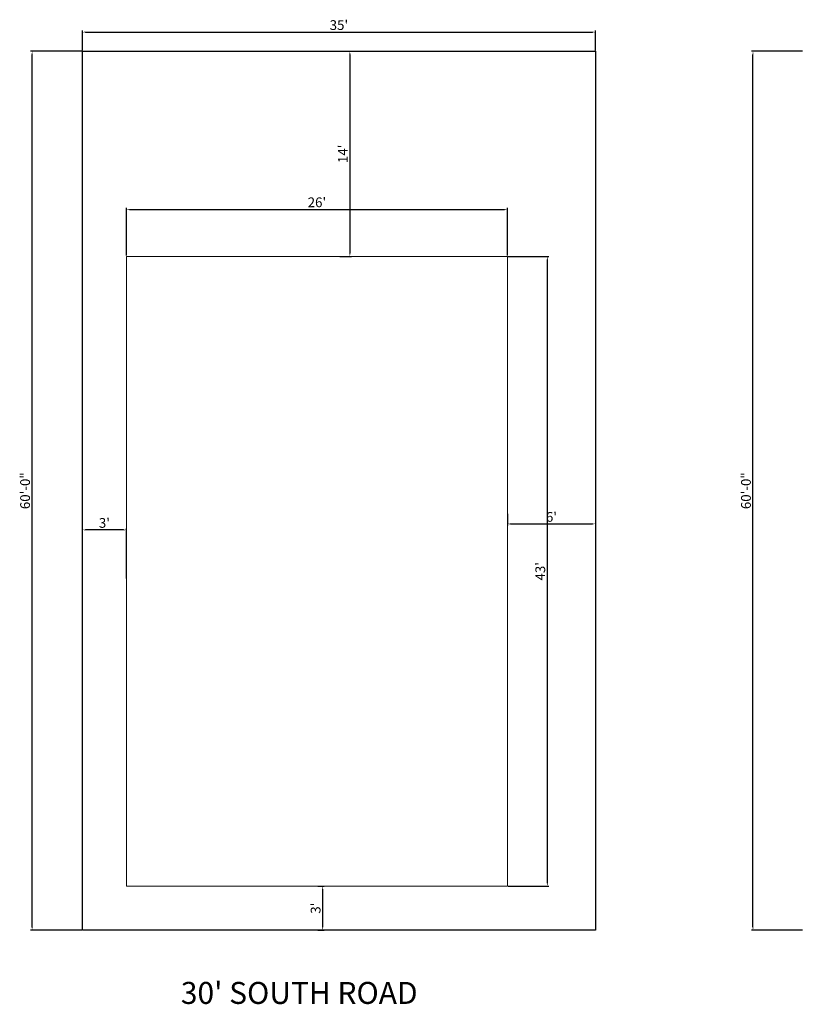
# Model space of a CAD drawing. Units: inches. Extents: x 538 to 2251, y 1112 to 1944.
# Tile 1 of 2: x 538 to 1179, y 1112 to 1918. Entities that reach past the tile are written whole.
import ezdxf

# ---------------------------------------------------------------- set-up
doc = ezdxf.new("R2010")
doc.units = ezdxf.units.IN
for name, color, linetype, lineweight in [('A-FLOR-OTLN', 7, 'Continuous', 18), ('C-PROP', 7, 'Continuous', 25), ('DIMENSIONS', 6, 'Continuous', 18), ('TEXT', 7, 'Continuous', 25)]:
    doc.layers.add(name, color=color, linetype=linetype, lineweight=lineweight)
doc.styles.get("Standard").update_dxf_attribs({"font": 'arial.ttf'})
doc.dimstyles.new('ISO-25', dxfattribs={"dimtxt": 8, "dimasz": 2.5, "dimexe": 1.25, "dimexo": 0.625, "dimtad": 1, "dimdec": 1, "dimlunit": 4, "dimtxsty": 'Standard', "dimcen": 2.5, "dimadec": 0, "dimazin": 0, "dimtfac": 1, "dimtdec": 1, "dimtmove": 0, "dimatfit": 3, "dimfxl": 1, "dimarcsym": 0})

# ---------------------------------------------------------------- blocks, each defined once
blk = doc.blocks.new('*D1')
at = {"layer": 'Defpoints', "color": 0, "transparency": 16777216}
for p in [(1008.95, 1908.31), (588.95, 1892.58), (1008.95, 1892.58)]:
    blk.add_point(p, dxfattribs=at)
at = {"layer": 'DIMENSIONS', "color": 0, "lineweight": -2, "transparency": 16777216}
for p, q in [((588.95, 1893.21), (588.95, 1909.56)), ((591.45, 1908.31), (1006.45, 1908.31)), ((1008.95, 1893.21), (1008.95, 1909.56))]:
    blk.add_line(p, q, dxfattribs=at)
at = {"layer": 'DIMENSIONS', "color": 0, "transparency": 16777216}
for points in [[(591.45, 1908.73), (591.45, 1907.9), (588.95, 1908.31)], [(1006.45, 1908.73), (1006.45, 1907.9), (1008.95, 1908.31)]]:
    blk.add_solid(points, dxfattribs=at)
at = {"layer": 'DIMENSIONS', "color": 0, "transparency": 16777216, "insert": (798.95, 1913.02), "char_height": 8, "attachment_point": 5}
blk.add_mtext("35'", dxfattribs=at)
blk = doc.blocks.new('*D2')
at = {"layer": 'Defpoints', "color": 0, "transparency": 16777216}
for p in [(936.95, 1763.11), (624.95, 1724.58), (936.95, 1724.58)]:
    blk.add_point(p, dxfattribs=at)
at = {"layer": 'DIMENSIONS', "color": 0, "lineweight": -2, "transparency": 16777216}
for p, q in [((624.95, 1725.21), (624.95, 1764.36)), ((627.45, 1763.11), (934.45, 1763.11)), ((936.95, 1725.21), (936.95, 1764.36))]:
    blk.add_line(p, q, dxfattribs=at)
at = {"layer": 'DIMENSIONS', "color": 0, "transparency": 16777216}
for points in [[(627.45, 1763.53), (627.45, 1762.69), (624.95, 1763.11)], [(934.45, 1763.53), (934.45, 1762.69), (936.95, 1763.11)]]:
    blk.add_solid(points, dxfattribs=at)
at = {"layer": 'DIMENSIONS', "color": 0, "transparency": 16777216, "insert": (780.95, 1767.82), "char_height": 8, "attachment_point": 5}
blk.add_mtext("26'", dxfattribs=at)
blk = doc.blocks.new('*D3')
at = {"layer": 'Defpoints', "color": 0, "transparency": 16777216}
for p in [(798.95, 1892.58), (798.95, 1724.58), (807.91, 1724.58)]:
    blk.add_point(p, dxfattribs=at)
at = {"layer": 'DIMENSIONS', "color": 0, "lineweight": -2, "transparency": 16777216}
for p, q in [((799.58, 1892.58), (809.16, 1892.58)), ((807.91, 1890.08), (807.91, 1727.08)), ((799.58, 1724.58), (809.16, 1724.58))]:
    blk.add_line(p, q, dxfattribs=at)
at = {"layer": 'DIMENSIONS', "color": 0, "transparency": 16777216}
for points in [[(807.49, 1890.08), (808.33, 1890.08), (807.91, 1892.58)], [(807.49, 1727.08), (808.33, 1727.08), (807.91, 1724.58)]]:
    blk.add_solid(points, dxfattribs=at)
at = {"layer": 'DIMENSIONS', "color": 0, "transparency": 16777216, "insert": (803.27, 1808.58), "char_height": 8, "attachment_point": 5, "rotation": 90}
blk.add_mtext("14'", dxfattribs=at)
blk = doc.blocks.new('*D4')
at = {"layer": 'Defpoints', "color": 0, "transparency": 16777216}
for p in [(936.95, 1514.21), (1008.95, 1514.21), (1008.95, 1505.41)]:
    blk.add_point(p, dxfattribs=at)
at = {"layer": 'DIMENSIONS', "color": 0, "lineweight": -2, "transparency": 16777216}
for p, q in [((936.95, 1513.59), (936.95, 1504.16)), ((1008.95, 1513.59), (1008.95, 1504.16)), ((939.45, 1505.41), (1006.45, 1505.41))]:
    blk.add_line(p, q, dxfattribs=at)
at = {"layer": 'DIMENSIONS', "color": 0, "transparency": 16777216}
for points in [[(939.45, 1505.82), (939.45, 1504.99), (936.95, 1505.41)], [(1006.45, 1505.82), (1006.45, 1504.99), (1008.95, 1505.41)]]:
    blk.add_solid(points, dxfattribs=at)
at = {"layer": 'DIMENSIONS', "color": 0, "transparency": 16777216, "insert": (972.95, 1510.11), "char_height": 8, "attachment_point": 5}
blk.add_mtext("6'", dxfattribs=at)
blk = doc.blocks.new('*D5')
at = {"layer": 'Defpoints', "color": 0, "transparency": 16777216}
for p in [(780.95, 1208.58), (780.95, 1172.58), (785.63, 1172.58)]:
    blk.add_point(p, dxfattribs=at)
at = {"layer": 'DIMENSIONS', "color": 0, "lineweight": -2, "transparency": 16777216}
for p, q in [((781.58, 1208.58), (786.88, 1208.58)), ((785.63, 1206.08), (785.63, 1175.08)), ((781.58, 1172.58), (786.88, 1172.58))]:
    blk.add_line(p, q, dxfattribs=at)
at = {"layer": 'DIMENSIONS', "color": 0, "transparency": 16777216}
for points in [[(785.21, 1206.08), (786.04, 1206.08), (785.63, 1208.58)], [(785.21, 1175.08), (786.04, 1175.08), (785.63, 1172.58)]]:
    blk.add_solid(points, dxfattribs=at)
at = {"layer": 'DIMENSIONS', "color": 0, "transparency": 16777216, "insert": (780.91, 1190.58), "char_height": 8, "attachment_point": 5, "rotation": 90}
blk.add_mtext("3'", dxfattribs=at)
blk = doc.blocks.new('*D6')
at = {"layer": 'Defpoints', "color": 0, "transparency": 16777216}
for p in [(588.95, 1500.48), (588.95, 1460.13), (624.95, 1460.13)]:
    blk.add_point(p, dxfattribs=at)
at = {"layer": 'DIMENSIONS', "color": 0, "lineweight": -2, "transparency": 16777216}
for p, q in [((588.95, 1460.76), (588.95, 1501.73)), ((622.45, 1500.48), (591.45, 1500.48)), ((624.95, 1460.76), (624.95, 1501.73))]:
    blk.add_line(p, q, dxfattribs=at)
at = {"layer": 'DIMENSIONS', "color": 0, "transparency": 16777216}
for points in [[(591.45, 1500.9), (591.45, 1500.07), (588.95, 1500.48)], [(622.45, 1500.9), (622.45, 1500.07), (624.95, 1500.48)]]:
    blk.add_solid(points, dxfattribs=at)
at = {"layer": 'DIMENSIONS', "color": 0, "transparency": 16777216, "insert": (606.95, 1505.19), "char_height": 8, "attachment_point": 5}
blk.add_mtext("3'", dxfattribs=at)
blk = doc.blocks.new('*D13')
at = {"layer": 'Defpoints', "color": 0, "transparency": 16777216}
for p in [(936.95, 1724.58), (936.95, 1208.58), (969.58, 1208.58)]:
    blk.add_point(p, dxfattribs=at)
at = {"layer": 'DIMENSIONS', "color": 0, "lineweight": -2, "transparency": 16777216}
for p, q in [((937.58, 1724.58), (970.83, 1724.58)), ((969.58, 1722.08), (969.58, 1211.08)), ((937.58, 1208.58), (970.83, 1208.58))]:
    blk.add_line(p, q, dxfattribs=at)
at = {"layer": 'DIMENSIONS', "color": 0, "transparency": 16777216}
for points in [[(969.16, 1722.08), (969.99, 1722.08), (969.58, 1724.58)], [(969.16, 1211.08), (969.99, 1211.08), (969.58, 1208.58)]]:
    blk.add_solid(points, dxfattribs=at)
at = {"layer": 'DIMENSIONS', "color": 0, "transparency": 16777216, "insert": (964.86, 1466.58), "char_height": 8, "attachment_point": 5, "rotation": 90}
blk.add_mtext("43'", dxfattribs=at)
blk = doc.blocks.new('*D39')
at = {"layer": 'Defpoints', "color": 0, "transparency": 16777216}
for p in [(547.75, 1892.58), (588.95, 1892.58), (588.95, 1172.58)]:
    blk.add_point(p, dxfattribs=at)
at = {"layer": 'DIMENSIONS', "color": 0, "lineweight": -2, "transparency": 16777216}
for p, q in [((588.33, 1892.58), (546.5, 1892.58)), ((547.75, 1175.08), (547.75, 1890.08)), ((588.33, 1172.58), (546.5, 1172.58))]:
    blk.add_line(p, q, dxfattribs=at)
at = {"layer": 'DIMENSIONS', "color": 0, "transparency": 16777216}
for points in [[(547.34, 1890.08), (548.17, 1890.08), (547.75, 1892.58)], [(547.34, 1175.08), (548.17, 1175.08), (547.75, 1172.58)]]:
    blk.add_solid(points, dxfattribs=at)
at = {"layer": 'DIMENSIONS', "color": 0, "transparency": 16777216, "insert": (543.04, 1532.58), "char_height": 8, "attachment_point": 5, "rotation": 90}
blk.add_mtext('60\'-0"', dxfattribs=at)
blk = doc.blocks.new('*D40')
at = {"layer": 'Defpoints', "color": 0, "transparency": 16777216}
for p in [(1137.98, 1892.58), (1179.18, 1892.58), (1179.18, 1172.58)]:
    blk.add_point(p, dxfattribs=at)
at = {"layer": 'DIMENSIONS', "color": 0, "lineweight": -2, "transparency": 16777216}
for p, q in [((1178.55, 1892.58), (1136.73, 1892.58)), ((1137.98, 1175.08), (1137.98, 1890.08)), ((1178.55, 1172.58), (1136.73, 1172.58))]:
    blk.add_line(p, q, dxfattribs=at)
at = {"layer": 'DIMENSIONS', "color": 0, "transparency": 16777216}
for points in [[(1137.56, 1890.08), (1138.39, 1890.08), (1137.98, 1892.58)], [(1137.56, 1175.08), (1138.39, 1175.08), (1137.98, 1172.58)]]:
    blk.add_solid(points, dxfattribs=at)
at = {"layer": 'DIMENSIONS', "color": 0, "transparency": 16777216, "insert": (1133.27, 1532.58), "char_height": 8, "attachment_point": 5, "rotation": 90}
blk.add_mtext('60\'-0"', dxfattribs=at)

msp = doc.modelspace()

# ---------------------------------------------------------------- linework, layer by layer
at = {"layer": 'A-FLOR-OTLN'}
for p, q in [((624.95, 1724.58), (936.95, 1724.58)), ((624.95, 1208.58), (624.95, 1724.58)), ((936.95, 1724.58), (936.95, 1208.58)), ((936.95, 1208.58), (624.95, 1208.58))]:
    msp.add_line(p, q, dxfattribs=at)
at = {"layer": 'C-PROP'}
for p, q in [((588.95, 1892.58), (1008.95, 1892.58)), ((588.95, 1172.58), (588.95, 1892.58)), ((1008.95, 1892.58), (1008.95, 1172.58)), ((1008.95, 1172.58), (588.95, 1172.58))]:
    msp.add_line(p, q, dxfattribs=at)

# ---------------------------------------------------------------- texts
at = {"layer": 'TEXT', "insert": (669.52, 1130.15), "char_height": 18, "attachment_point": 1}
msp.add_mtext_dynamic_manual_height_columns("30' SOUTH ROAD", width=205.0176, gutter_width=12.5, heights=[0], dxfattribs=at)

# ---------------------------------------------------------------- dimensions: what is measured, and where the dimension line sits
at = {"layer": 'DIMENSIONS'}
for base, p1, p2, picture, middle in [((1008.95, 1908.31), (588.95, 1892.58), (1008.95, 1892.58), '*D1', (798.95, 1913.02)), ((936.95, 1763.11), (624.95, 1724.58), (936.95, 1724.58), '*D2', (780.95, 1767.82)), ((588.95, 1500.48), (624.95, 1460.13), (588.95, 1460.13), '*D6', (606.95, 1505.19)), ((1008.95, 1505.41), (936.95, 1514.21), (1008.95, 1514.21), '*D4', (972.95, 1510.11))]:
    dim = msp.add_linear_dim(base=base, p1=p1, p2=p2, dimstyle='ISO-25', override={"dimclrd": 0, "dimclre": 0, "dimclrt": 0}, dxfattribs=at)
    dim.commit()
    dim.dimension.update_dxf_attribs({"geometry": picture, "text_midpoint": middle})
for base, p1, p2, override, picture, middle in [((547.75, 1892.58), (588.95, 1172.58), (588.95, 1892.58), {"dimdec": 1, "dimlfac": 1, "dimrnd": 0, "dimzin": 1, "dimdsep": 46, "dimlunit": 4, "dimfrac": 2}, '*D39', (543.04, 1532.58)), ((807.91, 1724.58), (798.95, 1892.58), (798.95, 1724.58), {"dimclrd": 0, "dimclre": 0, "dimclrt": 0}, '*D3', (803.27, 1808.58)), ((1137.98, 1892.58), (1179.18, 1172.58), (1179.18, 1892.58), {"dimdec": 1, "dimlfac": 1, "dimrnd": 0, "dimzin": 1, "dimdsep": 46, "dimlunit": 4, "dimfrac": 2}, '*D40', (1133.27, 1532.58)), ((969.58, 1208.58), (936.95, 1724.58), (936.95, 1208.58), {"dimclrd": 0, "dimclre": 0, "dimclrt": 0}, '*D13', (964.86, 1466.58)), ((785.63, 1172.58), (780.95, 1208.58), (780.95, 1172.58), {"dimclrd": 0, "dimclre": 0, "dimclrt": 0}, '*D5', (780.91, 1190.58))]:
    dim = msp.add_linear_dim(base=base, p1=p1, p2=p2, angle=90, dimstyle='ISO-25', override=override, dxfattribs=at)
    dim.commit()
    dim.dimension.update_dxf_attribs({"geometry": picture, "text_midpoint": middle})

doc.saveas('drawing.dxf')
